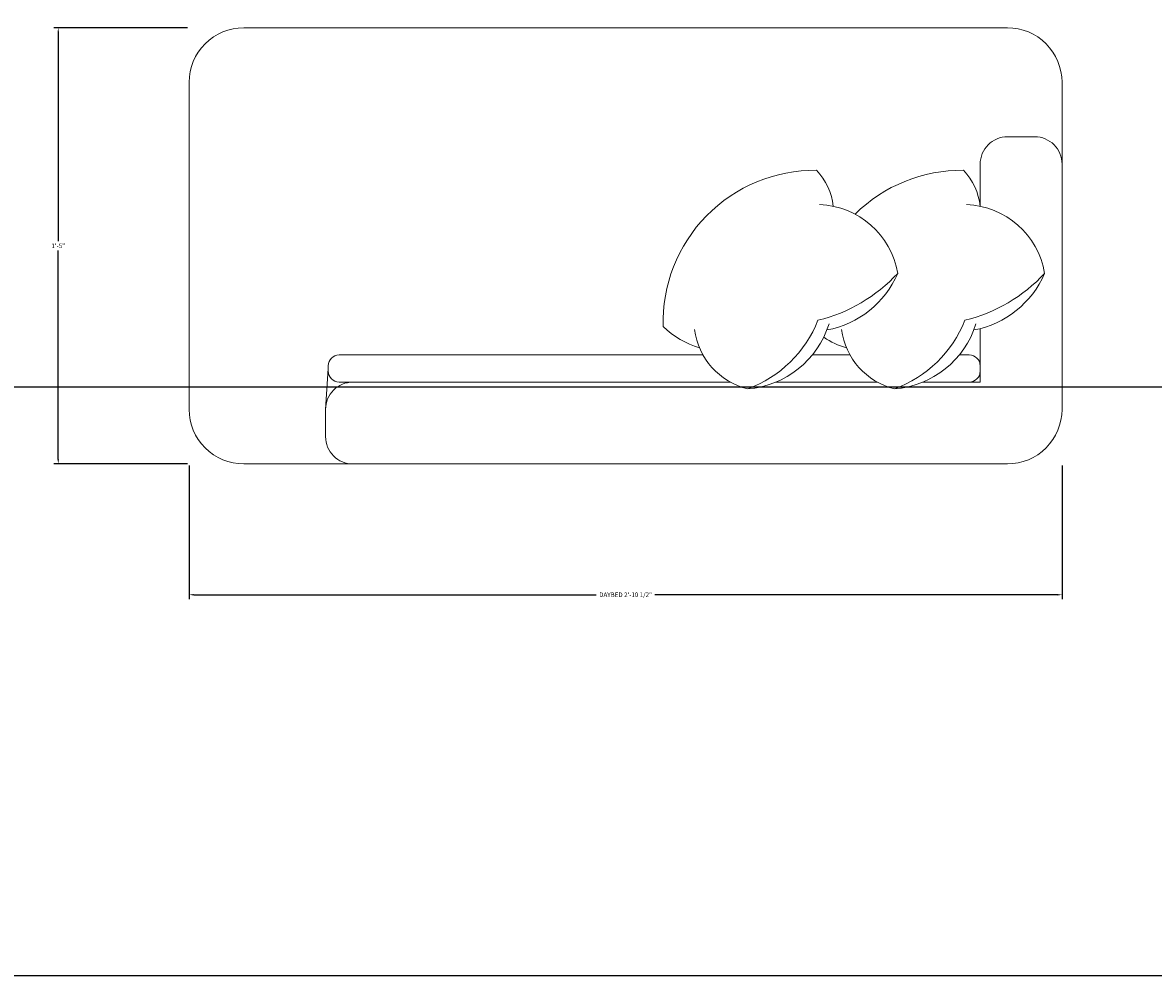
# Model space of a CAD drawing. Units: inches. Extents: x -5 to 330, y -522 to 40.
# Tile 16 of 23: x 201 to 246, y -417 to -380. Entities that reach past the tile are written whole.
import ezdxf

# ---------------------------------------------------------------- set-up
doc = ezdxf.new("R2010")
doc.units = ezdxf.units.IN
doc.header["$MEASUREMENT"] = 0
doc.layers.add('A-ANNO-DIMS', color=2, linetype='Continuous', lineweight=18)
doc.layers.add('A-FURN', color=8, linetype='Continuous', lineweight=18)
doc.styles.get("Standard").update_dxf_attribs({"font": 'arial.ttf'})
doc.dimstyles.get("Standard").update_dxf_attribs({"dimtxt": 0.18, "dimasz": 0.18, "dimexe": 0.18, "dimexo": 0.0625, "dimgap": 0.09, "dimtad": 0, "dimtih": 1, "dimtoh": 1, "dimdec": 0, "dimzin": 0, "dimdsep": 46, "dimlunit": 3, "dimtxsty": 'Standard', "dimcen": 0.09, "dimadec": 0, "dimazin": 0, "dimtfac": 1, "dimtdec": 0, "dimtofl": 0, "dimtmove": 0, "dimatfit": 3, "dimfxl": 1, "dimtolj": 1, "dimtzin": 0, "dimarcsym": 0})

# ---------------------------------------------------------------- blocks, each defined once
blk = doc.blocks.new('DAY BED1')
at = {"color": 0}
blk.add_line((0.3, 0.25), (0.225, 0.2549), dxfattribs=at)
blk.add_lwpolyline([(-0.3, 0, -0.414214), (-0.4, 0.1), (-0.4, 0.1, 0.317837), (-0.4, 0.1, -0.414214), (-0.4, 0.1), (-0.4, 0.1, 1.186185), (-0.4, 0.1, -0.414214), (-0.4, 0.1), (-0.4, 1.5, -0.414214), (-0.3, 1.6), (0.3, 1.6, -0.414214), (0.4, 1.5), (0.4, 0.1, -0.414214), (0.3, 0)], format="xyb", close=True, dxfattribs=at)
for points in [[(-0.0725, 1.45), (-0.15, 1.45, -0.414214), (-0.2, 1.5), (-0.2, 1.55, -0.414214), (-0.15, 1.6)], [(-0.0756, 1.4249, -0.356772), (0.0505, 1.5682, -0.249542), (0.1543, 1.4384, 9.61688)], [(0.0505, 1.5682, -0.14773), (0.1364, 1.422, -0.213343), (0.2624, 1.2931, -0.178662)], [(-0.0725, 1.4501, 0.165541), (-0.1386, 1.4192, 0.200231), (-0.0581, 1.2207, 0.121523)], [(0.1433, 1.4422, -0.306663), (0.2624, 1.2931, -0.30633), (0.1536, 1.1957, 0.872847)], [(0.25, 1.3448), (0.25, 1.45), (0.1517, 1.45, -0.414214)], [(0.2, 1.4118), (0.2, 1.43, -0.414214), (0.22, 1.45), (0.23, 1.45, -0.414214), (0.25, 1.43)], [(0.25, 1.43), (0.25, 1.3448, -0.414214)], [(-0.0756, 1.1556, -0.356772), (0.0505, 1.2988, -0.249542), (0.1543, 1.169, 9.61688)], [(0.0505, 1.2988, -0.14773), (0.1364, 1.1527, -0.213343), (0.2624, 1.0238, -0.178662)], [(0.25, 1.2616), (0.25, 1.0755, -0.414214)], [(0.1678, 1.1631, 0.071865), (0.1873, 1.205, -7.115464)], [(0.2, 1.1425), (0.2, 1.2113, -0.414214)], [(-0.0725, 1.1808, 0.165541), (-0.1386, 1.1498, 0.425989), (0.1479, 0.869, 0.121523), (0.1873, 0.9357, -7.115464)], [(0.1433, 1.1729, -0.306663), (0.2624, 1.0238, -0.30633), (0.1536, 0.9263, 0.872847)], [(0.25, 0.9923), (0.25, 0.2749, -0.414214), (0.23, 0.2549), (0.22, 0.2549, -0.414214), (0.2, 0.2749), (0.2, 0.9419, -0.414214)], [(0.25, 0.3775), (0.25, 0.3, 0.414214), (0.3, 0.25), (0.35, 0.25, 0.414214), (0.4, 0.3)]]:
    blk.add_lwpolyline(points, format="xyb", dxfattribs=at)
for points in [[(0.25, 1.0755), (0.25, 1.2616)], [(0.25, 0.3775), (0.25, 0.9923)]]:
    blk.add_lwpolyline(points, dxfattribs=at)
blk = doc.blocks.new('*D35')
at = {"layer": 'A-ANNO-DIMS', "color": 0, "lineweight": -2, "transparency": 16777216}
for p, q in [((207.497, -397.029), (207.497, -402.308)), ((241.908, -397.029), (241.908, -402.308)), ((207.677, -402.128), (223.546, -402.128)), ((241.728, -402.128), (225.859, -402.128))]:
    blk.add_line(p, q, dxfattribs=at)
at = {"layer": 'A-ANNO-DIMS', "color": 0, "transparency": 16777216}
for points in [[(207.677, -402.098), (207.677, -402.158), (207.497, -402.128)], [(241.728, -402.098), (241.728, -402.158), (241.908, -402.128)]]:
    blk.add_solid(points, dxfattribs=at)
at = {"layer": 'Defpoints', "color": 0, "transparency": 16777216}
for p in [(207.497, -396.967), (241.908, -396.967), (241.908, -402.128)]:
    blk.add_point(p, dxfattribs=at)
at = {"layer": 'A-ANNO-DIMS', "color": 0, "transparency": 16777216, "insert": (224.703, -402.128), "char_height": 0.18, "attachment_point": 5}
blk.add_mtext('\\A1;DAYBED 2\'-10 1/2"', dxfattribs=at)
blk = doc.blocks.new('*D36')
at = {"layer": 'A-ANNO-DIMS', "color": 0, "lineweight": -2, "transparency": 16777216}
for p, q in [((207.435, -379.762), (202.156, -379.762)), ((202.336, -379.942), (202.336, -388.182)), ((202.336, -396.787), (202.336, -388.546)), ((207.435, -396.967), (202.156, -396.967))]:
    blk.add_line(p, q, dxfattribs=at)
at = {"layer": 'A-ANNO-DIMS', "color": 0, "transparency": 16777216}
for points in [[(202.306, -379.942), (202.366, -379.942), (202.336, -379.762)], [(202.306, -396.787), (202.366, -396.787), (202.336, -396.967)]]:
    blk.add_solid(points, dxfattribs=at)
at = {"layer": 'Defpoints', "color": 0, "transparency": 16777216}
for p in [(207.497, -379.762), (202.336, -396.967), (207.497, -396.967)]:
    blk.add_point(p, dxfattribs=at)
at = {"layer": 'A-ANNO-DIMS', "color": 0, "transparency": 16777216, "insert": (202.336, -388.364), "char_height": 0.18, "attachment_point": 5}
blk.add_mtext('\\A1;1\'-5"', dxfattribs=at)
blk = doc.blocks.new('*D37')
at = {"layer": 'A-ANNO-DIMS', "color": 0, "lineweight": -2, "transparency": 16777216}
for p, q in [((164.01, -53.206), (164.01, -522.309)), ((272.01, -53.206), (272.01, -522.309)), ((164.19, -522.129), (217.681, -522.129)), ((271.83, -522.129), (218.339, -522.129))]:
    blk.add_line(p, q, dxfattribs=at)
at = {"layer": 'A-ANNO-DIMS', "color": 0, "transparency": 16777216}
for points in [[(164.19, -522.099), (164.19, -522.159), (164.01, -522.129)], [(271.83, -522.099), (271.83, -522.159), (272.01, -522.129)]]:
    blk.add_solid(points, dxfattribs=at)
at = {"layer": 'Defpoints', "color": 0, "transparency": 16777216}
for p in [(164.01, -53.144), (272.01, -53.144), (272.01, -522.129)]:
    blk.add_point(p, dxfattribs=at)
at = {"layer": 'A-ANNO-DIMS', "color": 0, "transparency": 16777216, "insert": (218.01, -522.129), "char_height": 0.18, "attachment_point": 5}
blk.add_mtext('\\A1;9\'-0"', dxfattribs=at)
blk = doc.blocks.new('*D44')
at = {"layer": 'A-ANNO-DIMS', "color": 0, "lineweight": -2, "transparency": 16777216}
for p, q in [((128.572, -393.928), (308.175, -393.928)), ((307.995, -394.108), (307.995, -405.356)), ((307.995, -416.964), (307.995, -405.716)), ((128.572, -417.144), (308.175, -417.144))]:
    blk.add_line(p, q, dxfattribs=at)
at = {"layer": 'A-ANNO-DIMS', "color": 0, "transparency": 16777216}
for points in [[(307.965, -394.108), (308.025, -394.108), (307.995, -393.928)], [(307.965, -416.964), (308.025, -416.964), (307.995, -417.144)]]:
    blk.add_solid(points, dxfattribs=at)
at = {"layer": 'Defpoints', "color": 0, "transparency": 16777216}
for p in [(128.51, -393.928), (307.995, -393.928), (128.51, -417.144)]:
    blk.add_point(p, dxfattribs=at)
at = {"layer": 'A-ANNO-DIMS', "color": 0, "transparency": 16777216, "insert": (307.995, -405.536), "char_height": 0.18, "attachment_point": 5}
blk.add_mtext('\\A1;1\'-11"', dxfattribs=at)

msp = doc.modelspace()

# ---------------------------------------------------------------- block references
at = {"layer": 'A-FURN', "ltscale": 0.03, "xscale": 21.50662746172407, "yscale": 21.50662746172407, "zscale": 21.50662746172407, "rotation": 270}
msp.add_blockref('DAY BED1', (207.497, -388.364), dxfattribs=at)

# ---------------------------------------------------------------- dimensions: what is measured, and where the dimension line sits
at = {"layer": 'A-ANNO-DIMS'}
dim = msp.add_linear_dim(base=(272.01, -522.129), p1=(164.01, -53.144), p2=(272.01, -53.144), dimstyle='Standard', override={"dimdec": 1, "dimlfac": 1, "dimrnd": 0, "dimzin": 1, "dimdsep": 46, "dimlunit": 4, "dimfrac": 2}, dxfattribs=at)
dim.commit()
dim.dimension.update_dxf_attribs({"geometry": '*D37', "text_midpoint": (218.01, -522.129)})
for base, p1, p2, angle, picture, middle in [((202.336, -396.967), (207.497, -379.762), (207.497, -396.967), 270, '*D36', (202.336, -388.364)), ((307.995, -393.928), (128.51, -417.144), (128.51, -393.928), 90, '*D44', (307.995, -405.536))]:
    dim = msp.add_linear_dim(base=base, p1=p1, p2=p2, angle=angle, dimstyle='Standard', override={"dimdec": 1, "dimlfac": 1, "dimrnd": 0, "dimzin": 1, "dimdsep": 46, "dimlunit": 4, "dimfrac": 2}, dxfattribs=at)
    dim.commit()
    dim.dimension.update_dxf_attribs({"geometry": picture, "text_midpoint": middle})
dim = msp.add_linear_dim(base=(241.908, -402.128), p1=(207.497, -396.967), p2=(241.908, -396.967), text='DAYBED <>', dimstyle='Standard', override={"dimdec": 1, "dimlfac": 1, "dimrnd": 0, "dimzin": 1, "dimdsep": 46, "dimlunit": 4, "dimfrac": 2}, dxfattribs=at)
dim.commit()
dim.dimension.update_dxf_attribs({"geometry": '*D35', "text_midpoint": (224.703, -402.128)})

doc.saveas('drawing.dxf')
